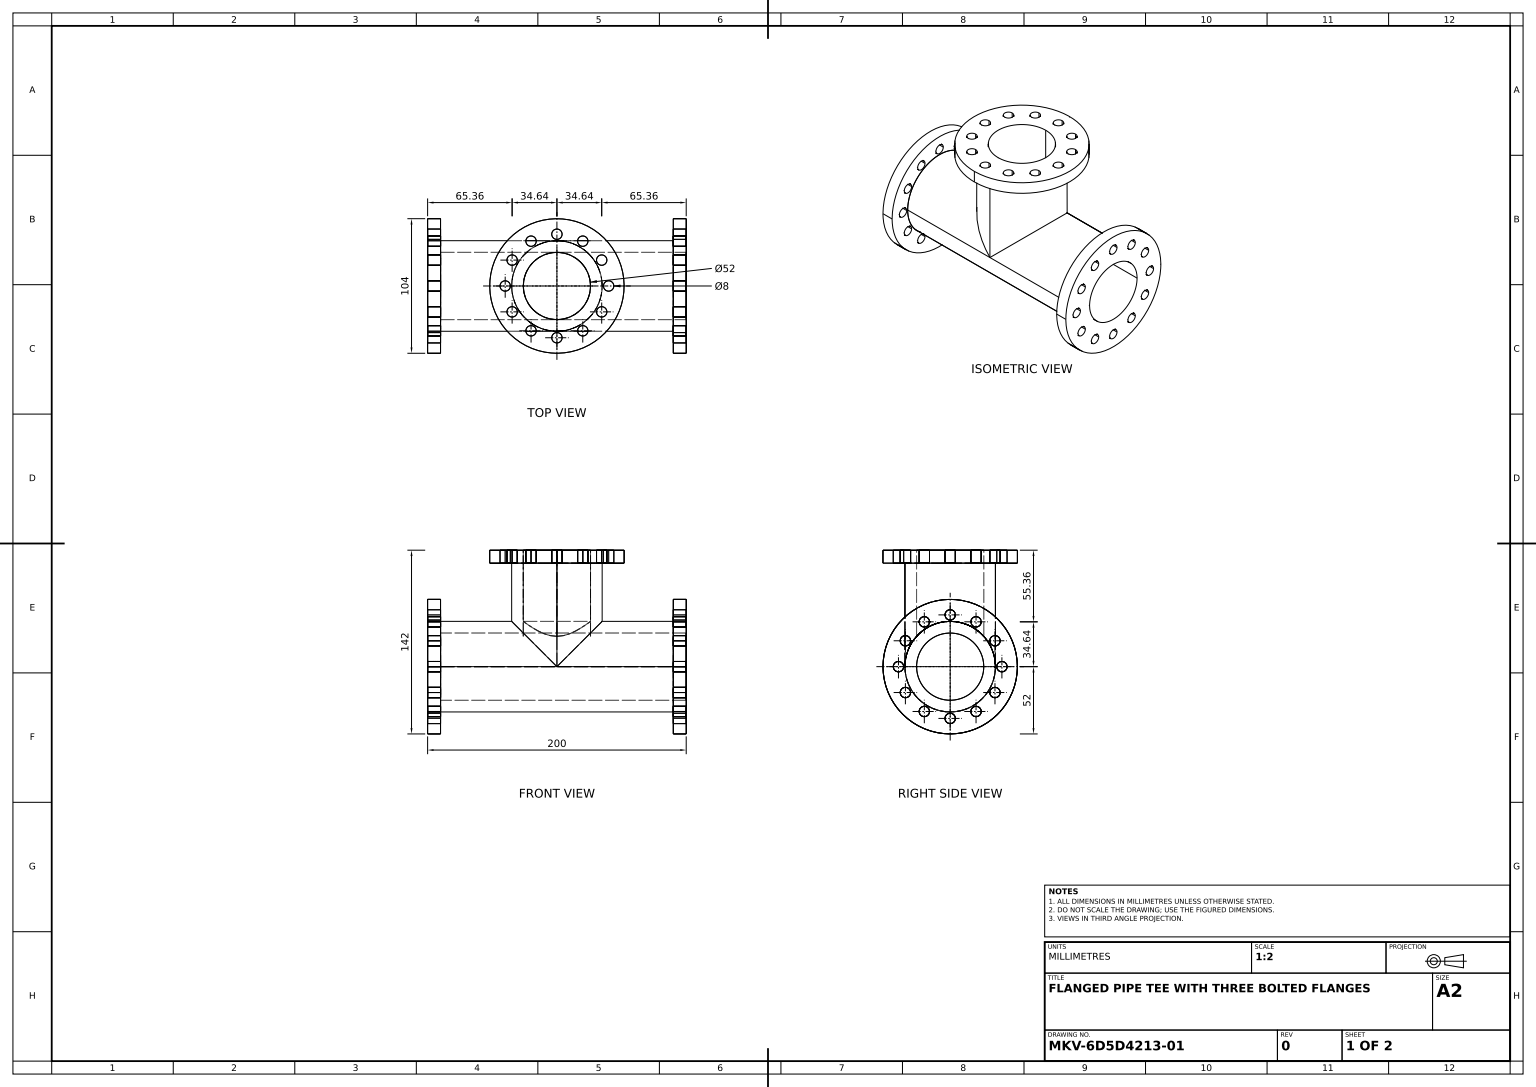
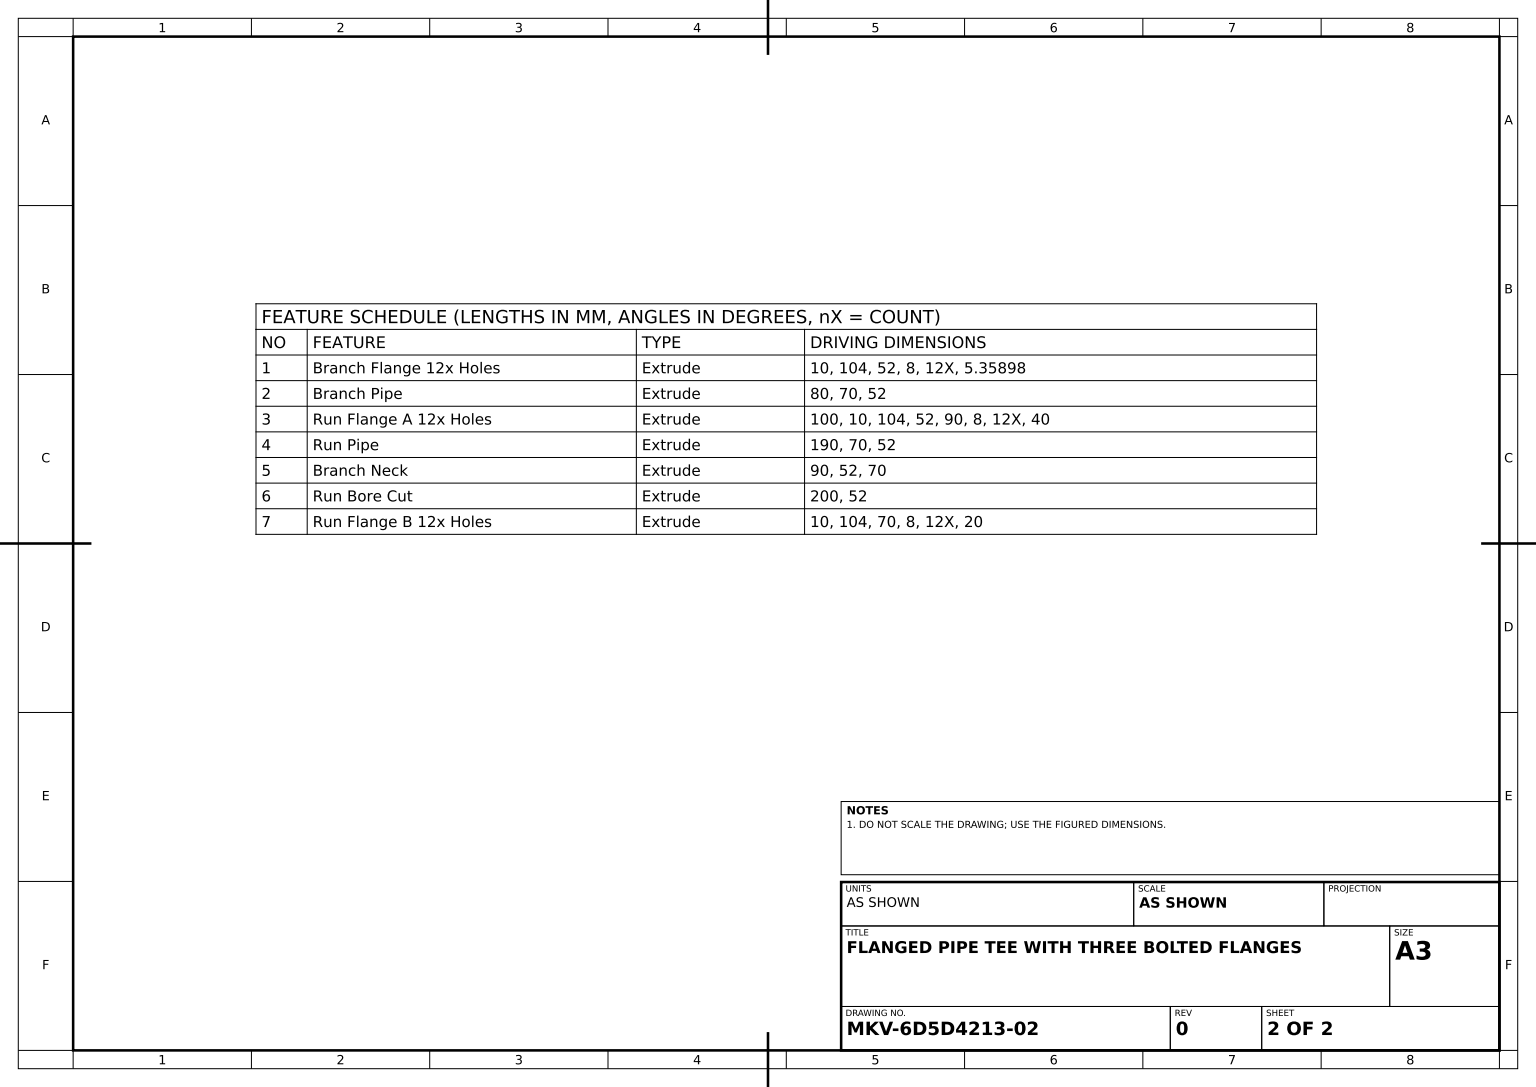
SolidWorks part; units mm, degrees
material "Plain Carbon Steel"
ref_plane "Front Plane" through (0, 0, 0) normal (0, 0, 1) x (1, 0, 0)
ref_plane "Top Plane" through (0, 0, 0) normal (0, 1, 0) x (1, 0, 0)
ref_plane "Right Plane" through (0, 0, 0) normal (1, 0, 0) x (0, 0, -1)
sketch "Branch Flange Profile" plane through (0, 0, 0) normal (0, 1, 0) x (1, 0, 0)
  circle A0 centre (0, 0) radius 52
  circle A1 centre (0, 0) radius 26
  circle A3 centre (0, 40) radius 4
  circle A4 centre (20, 34.641) radius 4
  circle A5 centre (34.641, 20) radius 4
  circle A6 centre (40, 0) radius 4
  circle A7 centre (34.641, -20) radius 4
  circle A8 centre (20, -34.641) radius 4
  circle A9 centre (0, -40) radius 4
  circle A10 centre (-20, -34.641) radius 4
  circle A11 centre (-34.641, -20) radius 4
  circle A12 centre (-40, 0) radius 4
  circle A13 centre (-34.641, 20) radius 4
  circle A14 centre (-20, 34.641) radius 4
  dimension "D1" = 104
  dimension "D2" = 52
  dimension "D3" = 5.359
  dimension "D4" = 8
  dimension "D5" = 12
extrude "Branch Flange 12x Holes" add sketch "Branch Flange Profile" against normal blind 10
sketch "Branch Pipe Profile" plane through (0, 0, 0) normal (0, 1, 0) x (1, 0, 0)
  circle A0 centre (0, 0) radius 26
  circle A1 centre (0, 0) radius 35
  dimension "D1" = 70
  dimension "D2" = 52
extrude "Branch Pipe" add sketch "Branch Pipe Profile" against normal blind 80
ref_plane "Run Flange A Plane" through (100, 0, 0) normal (1, 0, 0) x (0, 0, -1)
sketch "Run Flange A Profile" plane through (100, 0, 0) normal (1, 0, 0) x (0, 0, -1)
  circle A0 centre (0, -90) radius 52
  circle A1 centre (0, -90) radius 26
  circle A3 centre (0, -50) radius 4
  circle A4 centre (20, -55.359) radius 4
  circle A5 centre (34.641, -70) radius 4
  circle A6 centre (40, -90) radius 4
  circle A7 centre (34.641, -110) radius 4
  circle A8 centre (20, -124.641) radius 4
  circle A9 centre (0, -130) radius 4
  circle A10 centre (-20, -124.641) radius 4
  circle A11 centre (-34.641, -110) radius 4
  circle A12 centre (-40, -90) radius 4
  circle A13 centre (-34.641, -70) radius 4
  circle A14 centre (-20, -55.359) radius 4
  dimension "D1" = 40
  dimension "D2" = 104
  dimension "D3" = 52
  dimension "D5" = 8
  dimension "D4" = 90
  dimension "D6" = 12
extrude "Run Flange A 12x Holes" add sketch "Run Flange A Profile" against normal blind 10 separate body
sketch "Run Pipe Profile" plane through (100, 0, 0) normal (1, 0, 0) x (0, 0, -1)
  circle A0 centre (0, -90) radius 35
  circle A1 centre (0, -90) radius 26
  dimension "D1" = 70
  dimension "D2" = 52
extrude "Run Pipe" add sketch "Run Pipe Profile" against normal blind 190
sketch "Branch Neck Profile" plane through (0, 0, 0) normal (0, 1, 0) x (1, 0, 0)
  circle A0 centre (0, 0) radius 26
  circle A1 centre (0, 0) radius 35
  dimension "D1" = 52
  dimension "D2" = 70
extrude "Branch Neck" add sketch "Branch Neck Profile" against normal blind 90
sketch "Run Bore Profile" plane through (100, 0, 0) normal (1, 0, 0) x (0, 0, -1)
  circle A0 centre (0, -90) radius 26
  dimension "D1" = 52
extrude "Run Bore Cut" cut sketch "Run Bore Profile" against normal blind 200
sketch "Run Flange B Profile" plane through (-90, 0, 0) normal (-1, 0, 0) x (0, 0, 1)
  circle A0 centre (0, -90) radius 52
  circle A1 centre (0, -90) radius 35
  circle A3 centre (0, -50) radius 4
  circle A4 centre (20, -55.359) radius 4
  circle A5 centre (34.641, -70) radius 4
  circle A6 centre (40, -90) radius 4
  circle A7 centre (34.641, -110) radius 4
  circle A8 centre (20, -124.641) radius 4
  circle A9 centre (0, -130) radius 4
  circle A10 centre (-20, -124.641) radius 4
  circle A11 centre (-34.641, -110) radius 4
  circle A12 centre (-40, -90) radius 4
  circle A13 centre (-34.641, -70) radius 4
  circle A14 centre (-20, -55.359) radius 4
  circle A15 centre (0, -90) radius 26 construction
  dimension "D1" = 104
  dimension "D2" = 70
  dimension "D3" = 8
  dimension "D5" = 20
  dimension "D4" = 12
extrude "Run Flange B 12x Holes" add sketch "Run Flange B Profile" along normal blind 10 separate body
